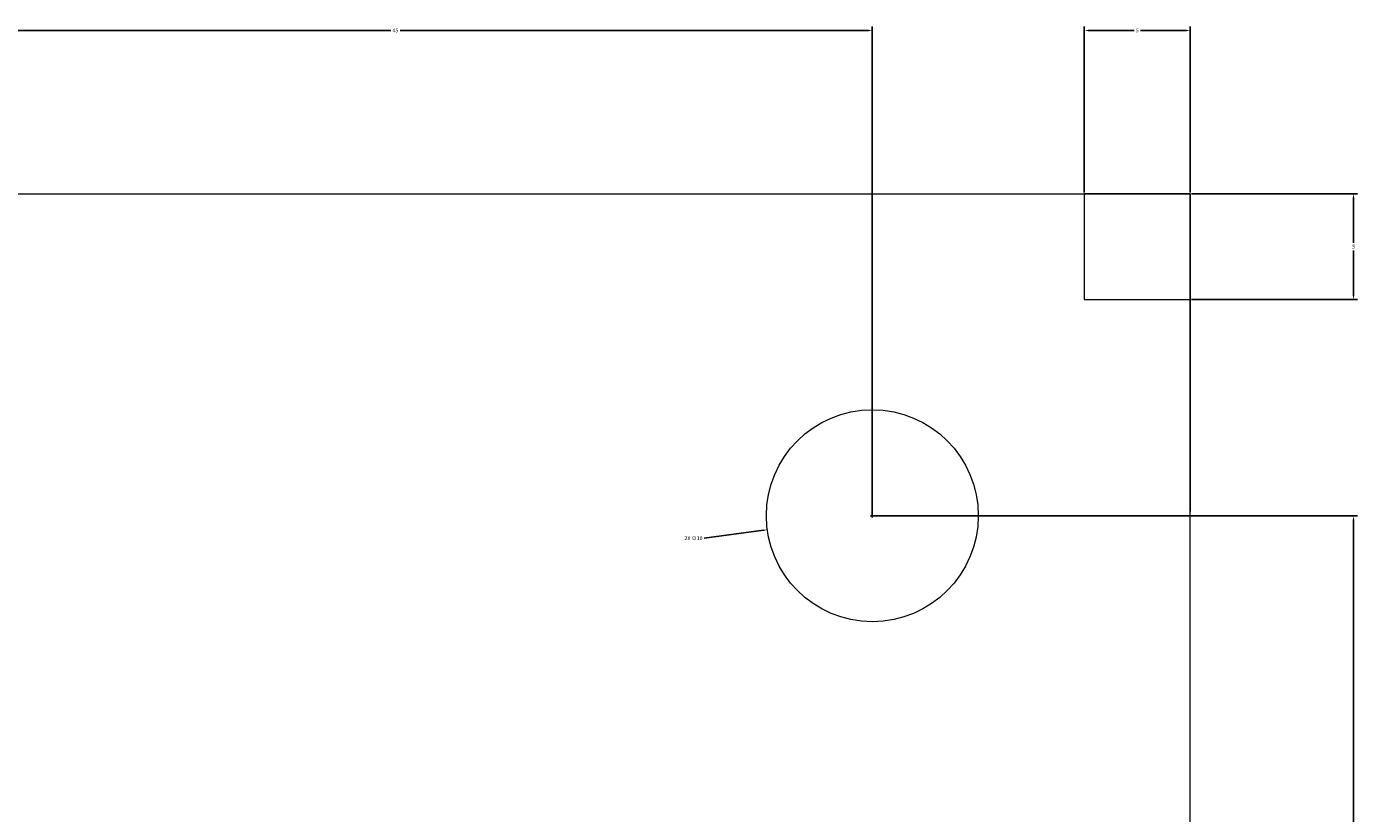
# Model space of a CAD drawing. Units: inches. Extents: x -19 to 107, y -27 to 49.
# Tile 4 of 4: x 44 to 107, y 12 to 49. Entities that reach past the tile are written whole.
import ezdxf

# ---------------------------------------------------------------- set-up
doc = ezdxf.new("R2010")
doc.units = ezdxf.units.IN
doc.header["$MEASUREMENT"] = 0
doc.layers.add('M-CONS', color=8, linetype='Continuous', lineweight=18)
doc.layers.add('M-DIMS', color=2, linetype='Continuous', lineweight=18)
doc.styles.get("Standard").update_dxf_attribs({"font": 'arial.ttf'})
doc.dimstyles.get("Standard").update_dxf_attribs({"dimtxt": 0.18, "dimasz": 0.18, "dimexe": 0.18, "dimexo": 0.0625, "dimgap": 0.09, "dimtad": 0, "dimtih": 1, "dimtoh": 1, "dimdec": 4, "dimzin": 0, "dimdsep": 46, "dimtxsty": 'Standard', "dimcen": 0.09, "dimadec": 0, "dimazin": 0, "dimtfac": 1, "dimtdec": 4, "dimtofl": 0, "dimtmove": 0, "dimatfit": 3, "dimfxl": 1, "dimtolj": 1, "dimtzin": 0, "dimarcsym": 0})

# ---------------------------------------------------------------- blocks, each defined once
blk = doc.blocks.new('*D4')
at = {"layer": 'Defpoints', "color": 0, "transparency": 16777216}
for p in [(84.063, 48.525), (39.063, 40.82), (84.063, 25.624)]:
    blk.add_point(p, dxfattribs=at)
at = {"layer": 'M-DIMS', "color": 0, "lineweight": -2, "transparency": 16777216}
for p, q in [((39.063, 40.883), (39.063, 48.705)), ((39.243, 48.525), (61.34, 48.525)), ((83.883, 48.525), (61.787, 48.525)), ((84.063, 25.687), (84.063, 48.705))]:
    blk.add_line(p, q, dxfattribs=at)
at = {"layer": 'M-DIMS', "color": 0, "transparency": 16777216}
for points in [[(39.243, 48.555), (39.243, 48.495), (39.063, 48.525)], [(83.883, 48.555), (83.883, 48.495), (84.063, 48.525)]]:
    blk.add_solid(points, dxfattribs=at)
at = {"layer": 'M-DIMS', "color": 0, "transparency": 16777216, "insert": (61.563, 48.525), "char_height": 0.18, "attachment_point": 5}
blk.add_mtext('\\A1;45', dxfattribs=at)
blk = doc.blocks.new('*D5')
at = {"layer": 'Defpoints', "color": 0, "transparency": 16777216}
for p in [(99.063, 48.525), (94.063, 40.82), (99.063, 40.82)]:
    blk.add_point(p, dxfattribs=at)
at = {"layer": 'M-DIMS', "color": 0, "lineweight": -2, "transparency": 16777216}
for p, q in [((94.063, 40.883), (94.063, 48.705)), ((94.243, 48.525), (96.414, 48.525)), ((98.883, 48.525), (96.713, 48.525)), ((99.063, 40.883), (99.063, 48.705))]:
    blk.add_line(p, q, dxfattribs=at)
at = {"layer": 'M-DIMS', "color": 0, "transparency": 16777216}
for points in [[(94.243, 48.555), (94.243, 48.495), (94.063, 48.525)], [(98.883, 48.555), (98.883, 48.495), (99.063, 48.525)]]:
    blk.add_solid(points, dxfattribs=at)
at = {"layer": 'M-DIMS', "color": 0, "transparency": 16777216, "insert": (96.563, 48.525), "char_height": 0.18, "attachment_point": 5}
blk.add_mtext('\\A1;5', dxfattribs=at)
blk = doc.blocks.new('*D6')
at = {"layer": 'Defpoints', "color": 0, "transparency": 16777216}
for p in [(99.063, 40.82), (106.768, 40.82), (99.063, 35.82)]:
    blk.add_point(p, dxfattribs=at)
at = {"layer": 'M-DIMS', "color": 0, "lineweight": -2, "transparency": 16777216}
for p, q in [((99.126, 40.82), (106.948, 40.82)), ((106.768, 40.64), (106.768, 38.502)), ((106.768, 36), (106.768, 38.138)), ((99.126, 35.82), (106.948, 35.82))]:
    blk.add_line(p, q, dxfattribs=at)
at = {"layer": 'M-DIMS', "color": 0, "transparency": 16777216}
for points in [[(106.738, 40.64), (106.798, 40.64), (106.768, 40.82)], [(106.738, 36), (106.798, 36), (106.768, 35.82)]]:
    blk.add_solid(points, dxfattribs=at)
at = {"layer": 'M-DIMS', "color": 0, "transparency": 16777216, "insert": (106.768, 38.32), "char_height": 0.18, "attachment_point": 5}
blk.add_mtext('\\A1;5', dxfattribs=at)
blk = doc.blocks.new('*D7')
at = {"layer": 'Defpoints', "color": 0, "transparency": 16777216}
for p in [(84.063, 25.624), (106.768, 25.624), (84.063, -4.376)]:
    blk.add_point(p, dxfattribs=at)
at = {"layer": 'M-DIMS', "color": 0, "lineweight": -2, "transparency": 16777216}
for p, q in [((84.126, 25.624), (106.948, 25.624)), ((106.768, 25.444), (106.768, 10.806)), ((106.768, -4.196), (106.768, 10.443)), ((84.126, -4.376), (106.948, -4.376))]:
    blk.add_line(p, q, dxfattribs=at)
at = {"layer": 'M-DIMS', "color": 0, "transparency": 16777216}
for points in [[(106.738, 25.444), (106.798, 25.444), (106.768, 25.624)], [(106.738, -4.196), (106.798, -4.196), (106.768, -4.376)]]:
    blk.add_solid(points, dxfattribs=at)
at = {"layer": 'M-DIMS', "color": 0, "transparency": 16777216, "insert": (106.768, 10.624), "char_height": 0.18, "attachment_point": 5}
blk.add_mtext('\\A1;30', dxfattribs=at)
blk = doc.blocks.new('*D12')
at = {"layer": 'Defpoints', "color": 0, "transparency": 16777216}
for p in [(89.019, 26.288), (79.108, 24.961)]:
    blk.add_point(p, dxfattribs=at)
at = {"layer": 'M-DIMS', "color": 0, "lineweight": -2, "transparency": 16777216}
for p, q in [((83.973, 25.624), (84.153, 25.624)), ((84.063, 25.534), (84.063, 25.714)), ((76.134, 24.563), (78.929, 24.937))]:
    blk.add_line(p, q, dxfattribs=at)
at = {"layer": 'M-DIMS', "color": 0, "transparency": 16777216}
blk.add_solid([(78.925, 24.967), (78.933, 24.907), (79.108, 24.961)], dxfattribs=at)
at = {"layer": 'M-DIMS', "color": 0, "transparency": 16777216, "insert": (75.628, 24.563), "char_height": 0.18, "attachment_point": 5}
blk.add_mtext('\\A1;2X ∅10', dxfattribs=at)

msp = doc.modelspace()

# ---------------------------------------------------------------- linework, layer by layer
at = {"layer": 'M-CONS'}
for p, q in [((19.0635, 40.82), (99.0635, 40.82)), ((99.0635, -19.18), (99.0635, 40.82)), ((99.0635, 40.82), (99.0635, 25.82))]:
    msp.add_line(p, q, dxfattribs=at)
at = {"layer": 'M-CONS', "elevation": 20}
msp.add_lwpolyline([(99.0635, 40.82), (94.0635, 40.82), (94.0635, 35.82), (99.0635, 35.82)], close=True, dxfattribs=at)
at = {"layer": 'M-CONS'}
msp.add_circle((84.0635, 25.6245, 45), 5, dxfattribs=at)

# ---------------------------------------------------------------- dimensions: what is measured, and where the dimension line sits
at = {"layer": 'M-DIMS'}
for base, p1, p2, picture, middle in [((84.0635, 48.525), (39.0635, 40.82), (84.0635, 25.6245), '*D4', (61.5635, 48.525)), ((99.0635, 48.525), (94.0635, 40.82), (99.0635, 40.82), '*D5', (96.5635, 48.525))]:
    dim = msp.add_linear_dim(base=base, p1=p1, p2=p2, dimstyle='Standard', override={"dimdec": 0, "dimlfac": 1, "dimrnd": 0, "dimzin": 0, "dimdsep": 46, "dimlunit": 2}, dxfattribs=at)
    dim.commit()
    dim.dimension.update_dxf_attribs({"geometry": picture, "text_midpoint": middle})
for base, p1, p2, picture, middle in [((106.7685, 40.82), (99.0635, 35.82), (99.0635, 40.82), '*D6', (106.7685, 38.32)), ((106.7685, 25.6245), (84.0635, -4.3755), (84.0635, 25.6245), '*D7', (106.7685, 10.6245))]:
    dim = msp.add_linear_dim(base=base, p1=p1, p2=p2, angle=90, dimstyle='Standard', override={"dimdec": 0, "dimlfac": 1, "dimrnd": 0, "dimzin": 0, "dimdsep": 46, "dimlunit": 2}, dxfattribs=at)
    dim.commit()
    dim.dimension.update_dxf_attribs({"geometry": picture, "text_midpoint": middle})
dim = msp.add_diameter_dim_2p(p1=(89.0193, 26.2879), p2=(79.1077, 24.961), text='2X <>', dimstyle='Standard', override={"dimdec": 0, "dimlfac": 1, "dimrnd": 0, "dimzin": 0, "dimdsep": 46, "dimlunit": 2}, dxfattribs=at)
dim.commit()
dim.dimension.update_dxf_attribs({"geometry": '*D12', "text_midpoint": (76.1342, 24.563), "dimtype": 163})

doc.saveas('drawing.dxf')
